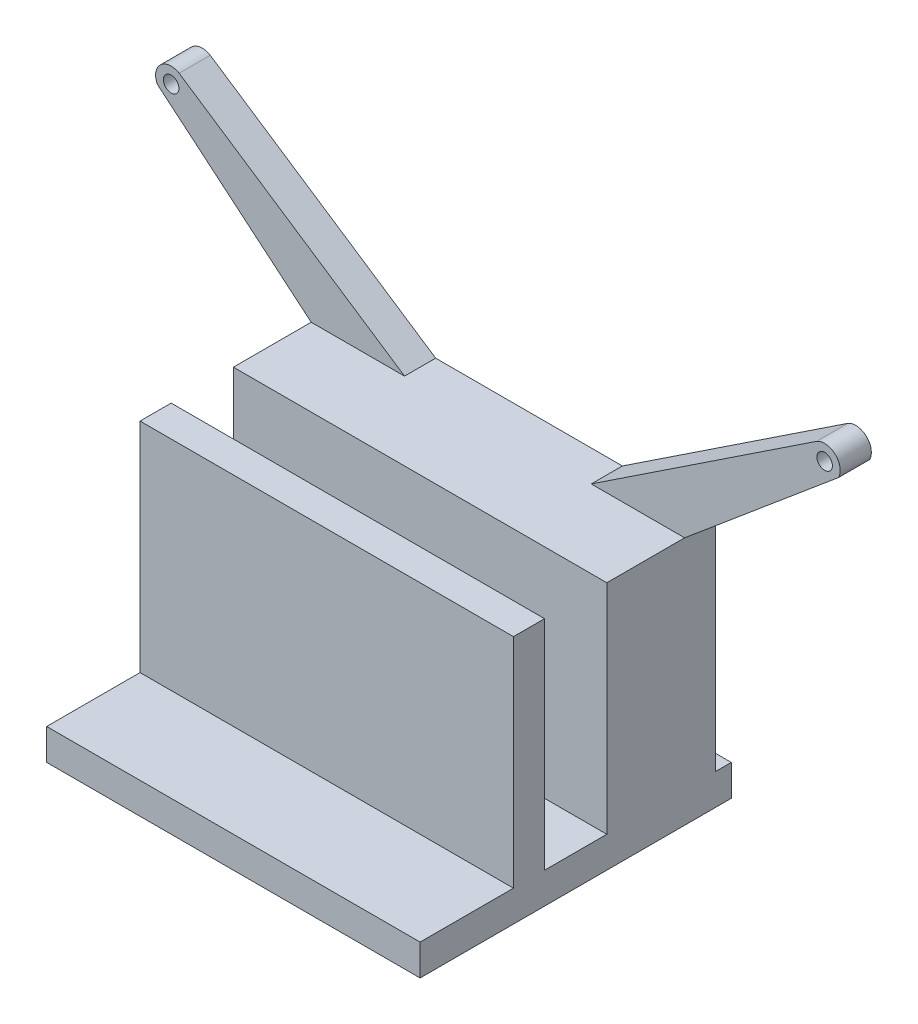
from build123d import *

# Parameters (mm, degrees)
SIDE_PROFILE_SKETCH_W            = 120
SIDE_PROFILE_SKETCH_H            = 10
MAIN_BODY_EXTRUDE_100_DEPTH      = 100
UPRIGHT_START                    = 5
SKETCH1_5_R                      = 2.5
SKETCH1_5_W                      = 120
SKETCH1_5_H                      = 80
SKETCH1_5_R_2                    = 4
UPRIGHT_BLOCK_EXTRUDE_35_DEPTH   = 35
FRONT_START                      = 5
SKETCH1_6_R                      = 2.5
FRONT_LEVER_ARM_EXTRUDE_10_DEPTH = 10
REAR_START                       = 60
SKETCH1_7_W                      = 120
SKETCH1_7_H                      = 70
REAR_LEVER_ARM_EXTRUDE_10_DEPTH  = 10


with BuildPart() as part:
    # Side Profile Sketch → Main Body Extrude 100 (new body)
    with BuildSketch(Plane.XY):
        with Locations((0, -35)):
            Rectangle(SIDE_PROFILE_SKETCH_W, SIDE_PROFILE_SKETCH_H)
    extrude(amount=MAIN_BODY_EXTRUDE_100_DEPTH)

    # Sketch1_5 → Upright Block Extrude 35 (add)
    # profile 1 of 3: a face of its own
    with BuildSketch(Plane.XY.offset(UPRIGHT_START)):
        with Locations((-105, 83.784559584)):
            Circle(SKETCH1_5_R)
    # profile 2 of 3: a face of its own
    with BuildSketch(Plane.XY.offset(UPRIGHT_START)):
        with Locations((105, 83.784559584)):
            Circle(SKETCH1_5_R)
    # profile 3 of 3: a face of its own
    with BuildSketch(Plane.XY.offset(UPRIGHT_START)):
        Rectangle(SKETCH1_5_W, SKETCH1_5_H)
        with Locations((-30, 0)):
            Circle(SKETCH1_5_R_2, mode=Mode.SUBTRACT)
        with Locations((30, 0)):
            Circle(SKETCH1_5_R_2, mode=Mode.SUBTRACT)
    extrude(amount=UPRIGHT_BLOCK_EXTRUDE_35_DEPTH)


with BuildPart() as upright_block_extrude_35_kept_piece:
    # of the separate pieces the step leaves, the one the design keeps (upright_block_extrude_35_pieces_kept)
    add(part.part.solids().sort_by_distance((60, -30, 0))[0])

    # Sketch1_6 → Front Lever Arm Extrude 10 (add)
    # profile 1 of 2: a face of its own
    with BuildSketch(Plane.XY.offset(FRONT_START)):
        with BuildLine():
            Line((102.433113428, 88.075374579), (30, 40))
            Line((30, 40), (60, 40))
            Line((60, 40), (109.439765001, 81.484888578))
            ThreePointArc((109.439765001, 81.484888578), (108.425718149, 87.426599557), (102.433113428, 88.075374579))
        make_face()
        with Locations((105, 83.784559584)):
            Circle(SKETCH1_6_R, mode=Mode.SUBTRACT)
    # profile 2 of 2: a face of its own
    with BuildSketch(Plane.XY.offset(FRONT_START)):
        with BuildLine():
            Line((-109.439765001, 81.484888578), (-60, 40))
            Line((-60, 40), (-30, 40))
            Line((-30, 40), (-102.433113428, 88.075374579))
            ThreePointArc((-102.433113428, 88.075374579), (-108.425718149, 87.426599557), (-109.439765001, 81.484888578))
        make_face()
        with Locations((-105, 83.784559584)):
            Circle(SKETCH1_6_R, mode=Mode.SUBTRACT)
    extrude(amount=FRONT_LEVER_ARM_EXTRUDE_10_DEPTH)

    # Sketch1_7 → Rear Lever Arm Extrude 10 (add)
    with BuildSketch(Plane.XY.offset(REAR_START)):
        with Locations((0, 5)):
            Rectangle(SKETCH1_7_W, SKETCH1_7_H)
    extrude(amount=REAR_LEVER_ARM_EXTRUDE_10_DEPTH)


solid = upright_block_extrude_35_kept_piece.part
